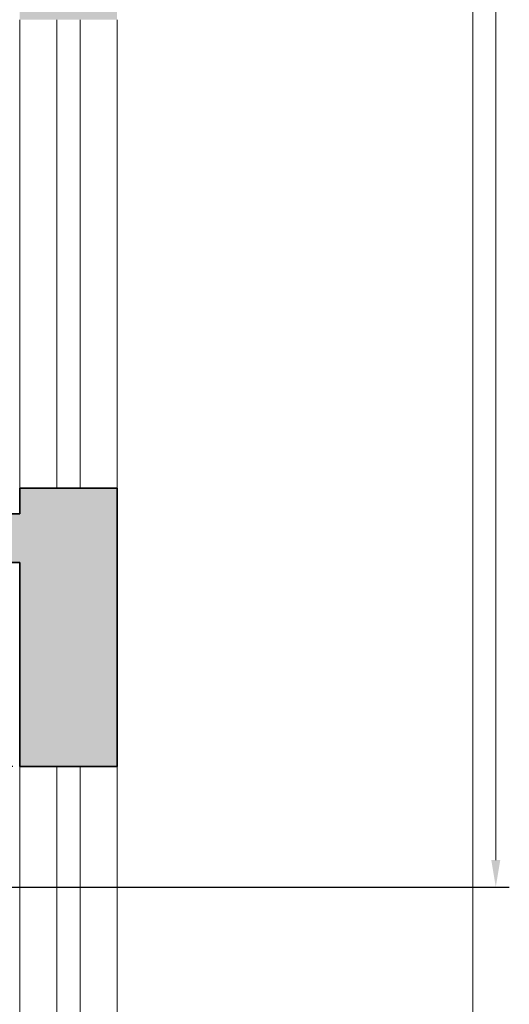
# Model space of a CAD drawing. Units: inches. Extents: x 2696 to 3240, y 1564 to 2310.
# Tile 37 of 76: x 3191 to 3236, y 1654 to 1745. Entities that reach past the tile are written whole.
import ezdxf

# ---------------------------------------------------------------- set-up
doc = ezdxf.new("R2010")
doc.units = ezdxf.units.IN
for name, color, linetype, lineweight in [('A-ANNO-DIMS', 3, 'Continuous', 18), ('A-WALL', 7, 'Continuous', 35), ('A-WALL-PATT', 9, 'Continuous', 13), ('WINDOW', 2, 'Continuous', 18)]:
    doc.layers.add(name, color=color, linetype=linetype, lineweight=lineweight)
doc.styles.add('TIMES NEW', font='times.ttf')
doc.dimstyles.new('Siddhuu', dxfattribs={"dimtxt": 6, "dimasz": 2.5, "dimexe": 1.25, "dimexo": 0.625, "dimtad": 1, "dimdec": 1, "dimlunit": 4, "dimtxsty": 'TIMES NEW', "dimcen": 2.5, "dimclrd": 256, "dimclre": 1, "dimclrt": 7, "dimadec": 0, "dimazin": 0, "dimtfac": 1, "dimtdec": 1, "dimtmove": 0, "dimatfit": 3, "dimfxl": 1, "dimtolj": 1, "dimlwd": -1, "dimarcsym": 0})

# ---------------------------------------------------------------- blocks, each defined once
blk = doc.blocks.new('WD_WIN4')
for p, q in [((-0.5, 0.5), (0.5, 0.5)), ((-0.5, 0.12), (0.5, 0.12)), ((-0.5, -0.12), (0.5, -0.12)), ((-0.5, -0.5), (0.5, -0.5))]:
    blk.add_line(p, q)
blk = doc.blocks.new('*D10')
at = {"layer": 'A-ANNO-DIMS', "color": 0, "lineweight": -2, "transparency": 16777216}
for p, q in [((3200.236, 2262.201), (3233.745, 2262.201)), ((3200.236, 1605.201), (3233.745, 1605.201))]:
    blk.add_line(p, q, dxfattribs=at)
at = {"layer": 'A-ANNO-DIMS', "color": 0, "transparency": 16777216}
blk.add_line((3232.495, 2250.201), (3232.495, 1617.201), dxfattribs=at)
for points in [[(3230.495, 2250.201), (3234.495, 2250.201), (3232.495, 2262.201)], [(3230.495, 1617.201), (3234.495, 1617.201), (3232.495, 1605.201)]]:
    blk.add_solid(points, dxfattribs=at)
at = {"layer": 'Defpoints', "color": 0, "transparency": 16777216}
for p in [(3199.611, 2262.201), (3199.611, 1605.201), (3232.495, 1605.201)]:
    blk.add_point(p, dxfattribs=at)
at = {"layer": 'A-ANNO-DIMS', "color": 0, "transparency": 16777216, "insert": (3222.714, 1933.701), "char_height": 18, "attachment_point": 5, "rotation": 90, "style": 'TIMES NEW'}
blk.add_mtext("\\A1;54'", dxfattribs=at)
blk = doc.blocks.new('*D26')
at = {"layer": 'A-ANNO-DIMS', "transparency": 16777216}
for p, q in [((3184.115, 1676.355), (3184.115, 1772.168)), ((3184.115, 1635.548), (3184.115, 1673.855))]:
    blk.add_line(p, q, dxfattribs=at)
at = {"layer": 'A-ANNO-DIMS', "color": 1, "lineweight": -2, "transparency": 16777216}
for p, q in [((3189.986, 1676.355), (3182.865, 1676.355)), ((3189.986, 1633.048), (3182.865, 1633.048))]:
    blk.add_line(p, q, dxfattribs=at)
at = {"layer": 'A-ANNO-DIMS', "transparency": 16777216}
for points in [[(3183.699, 1673.855), (3184.532, 1673.855), (3184.115, 1676.355)], [(3183.699, 1635.548), (3184.532, 1635.548), (3184.115, 1633.048)]]:
    blk.add_solid(points, dxfattribs=at)
at = {"layer": 'Defpoints', "color": 0, "transparency": 16777216}
for p in [(3184.115, 1676.355), (3190.611, 1676.355), (3190.611, 1633.048)]:
    blk.add_point(p, dxfattribs=at)
at = {"layer": 'A-ANNO-DIMS', "color": 7, "transparency": 16777216, "insert": (3180.348, 1725.511), "char_height": 6, "attachment_point": 5, "rotation": 90, "style": 'TIMES NEW'}
blk.add_mtext('\\A1;WINDOW 3\'-7 1/2" TYP.', dxfattribs=at)
blk = doc.blocks.new('*D56')
at = {"layer": 'A-ANNO-DIMS', "color": 1, "lineweight": -2, "transparency": 16777216}
for p, q in [((2966.334, 1884.201), (3235.861, 1884.201)), ((2966.334, 1665.201), (3235.861, 1665.201))]:
    blk.add_line(p, q, dxfattribs=at)
at = {"layer": 'A-ANNO-DIMS', "transparency": 16777216}
blk.add_line((3234.611, 1667.701), (3234.611, 1881.701), dxfattribs=at)
for points in [[(3234.195, 1881.701), (3235.028, 1881.701), (3234.611, 1884.201)], [(3234.195, 1667.701), (3235.028, 1667.701), (3234.611, 1665.201)]]:
    blk.add_solid(points, dxfattribs=at)
at = {"layer": 'Defpoints', "color": 0, "transparency": 16777216}
for p in [(2965.709, 1884.201), (3234.611, 1884.201), (2965.709, 1665.201)]:
    blk.add_point(p, dxfattribs=at)
at = {"layer": 'A-ANNO-DIMS', "color": 7, "transparency": 16777216, "insert": (3230.934, 1774.701), "char_height": 6, "attachment_point": 5, "rotation": 90, "style": 'TIMES NEW'}
blk.add_mtext('\\A1;18\'-3"', dxfattribs=at)

msp = doc.modelspace()

# ---------------------------------------------------------------- hatches: boundary and pattern name
at = {"layer": 'A-WALL-PATT', "transparency": 33554556}
h = msp.add_hatch(color=256, dxfattribs=at)
h.dxf.hatch_style = 1
h.paths.add_polyline_path([(2879.111, 2253.201), (2905.91, 2253.201), (2905.91, 2262.201), (2841.889, 2262.201), (2841.889, 2253.201), (2870.111, 2253.201), (2870.111, 2176.601), (2965.709, 2176.601), (2965.709, 2206.701), (2973.583, 2206.701), (2973.583, 2215.701), (2965.709, 2215.701), (2965.709, 2262.201), (2929.91, 2262.201), (2929.91, 2253.201), (2956.709, 2253.201), (2956.709, 2185.601), (2879.111, 2185.601)])
h.paths.add_polyline_path([(2782.834, 2262.201), (2745.611, 2262.201), (2745.611, 2228.729), (2754.611, 2228.729), (2754.611, 2253.201), (2782.834, 2253.201)])
h.paths.add_polyline_path([(2754.611, 2136.201), (2965.709, 2136.201), (2965.709, 2145.201), (2879.111, 2145.201), (2879.111, 2147.074), (2877.34, 2147.074), (2870.111, 2147.074), (2870.111, 2145.201), (2754.611, 2145.201), (2754.611, 2169.674), (2745.611, 2169.674), (2745.611, 2000.201), (2754.611, 2000.201), (2754.611, 2019.201), (2849.083, 2019.201), (2849.083, 2023.701), (2841.209, 2023.701), (2841.209, 2051.827), (2836.709, 2051.827), (2836.709, 2023.701), (2754.611, 2023.701), (2754.611, 2091.201), (2836.709, 2091.201), (2836.709, 2087.827), (2841.209, 2087.827), (2841.209, 2095.701), (2754.611, 2095.701)])
h.paths.add_polyline_path([(2965.709, 2136.201), (2956.709, 2136.201), (2956.709, 2023.701), (2885.083, 2023.701), (2885.083, 2019.201), (2956.709, 2019.201), (2956.709, 1950.575), (2965.709, 1950.575), (2965.709, 1980.201), (2973.583, 1980.201), (2973.583, 1989.201), (2965.709, 1989.201)])
h.paths.add_polyline_path([(2754.611, 1906.701), (2880.209, 1906.701), (2884.709, 1906.701), (2956.709, 1906.701), (2956.709, 1792.701), (2944.709, 1792.701), (2944.709, 1783.701), (2956.709, 1783.701), (2956.709, 1740.201), (2884.709, 1740.201), (2884.709, 1783.701), (2896.709, 1783.701), (2896.709, 1792.701), (2884.709, 1792.701), (2884.709, 1846.701), (2880.209, 1846.701), (2880.209, 1740.201), (2754.611, 1740.201), (2754.611, 1777.201), (2745.611, 1777.201), (2745.611, 1692.701), (2754.611, 1692.701), (2754.611, 1731.201), (2956.709, 1731.201), (2956.709, 1723.327), (2965.709, 1723.327), (2965.709, 1884.201), (2973.583, 1884.201), (2973.583, 1893.201), (2965.709, 1893.201), (2965.709, 1914.575), (2956.709, 1914.575), (2956.709, 1911.201), (2754.611, 1911.201), (2754.611, 1930.201), (2745.611, 1930.201), (2745.611, 1817.201), (2754.611, 1817.201), (2754.611, 1854.201), (2826.611, 1854.201), (2826.611, 1868.827), (2822.111, 1868.827), (2822.111, 1858.701), (2754.611, 1858.701)])
h.paths.add_polyline_path([(2965.709, 1656.201), (3008.237, 1656.201), (3008.237, 1665.201), (2965.709, 1665.201), (2965.709, 1693.327), (2956.709, 1693.327), (2956.709, 1686.201), (2934.583, 1686.201), (2934.583, 1681.701), (2956.709, 1681.701), (2956.709, 1614.201), (2896.709, 1614.201), (2896.709, 1681.701), (2904.583, 1681.701), (2904.583, 1686.201), (2892.209, 1686.201), (2892.209, 1614.201), (2858.41, 1614.201), (2858.41, 1605.201), (2965.709, 1605.201)])
h.paths.add_polyline_path([(2788.41, 1614.201), (2754.611, 1614.201), (2754.611, 1652.701), (2745.611, 1652.701), (2745.611, 1605.201), (2788.41, 1605.201)])
h.paths.add_polyline_path([(3199.611, 1633.048), (3190.611, 1633.048), (3190.611, 1614.201), (3082.611, 1614.201), (3082.611, 1665.201), (3070.237, 1665.201), (3070.237, 1656.201), (3078.111, 1656.201), (3078.111, 1605.201), (3199.611, 1605.201)])
h.paths.add_polyline_path([(3199.611, 1702.048), (3190.611, 1702.048), (3190.611, 1699.701), (3106.611, 1699.701), (3106.611, 1747.701), (3190.611, 1747.701), (3190.611, 1752.201), (3082.611, 1752.201), (3082.611, 1760.075), (3078.111, 1760.075), (3078.111, 1747.701), (3102.111, 1747.701), (3102.111, 1699.701), (3078.111, 1699.701), (3078.111, 1695.201), (3190.611, 1695.201), (3190.611, 1676.355), (3199.611, 1676.355)])
h.paths.add_polyline_path([(3199.611, 1783.201), (3190.611, 1783.201), (3190.611, 1745.355), (3199.611, 1745.355)])
h.paths.add_polyline_path([(3082.611, 1884.201), (3190.611, 1884.201), (3190.611, 1853.201), (3199.611, 1853.201), (3199.611, 1901.701), (3190.611, 1901.701), (3190.611, 1893.201), (3005.583, 1893.201), (3005.583, 1891.281), (3005.583, 1884.201), (3078.111, 1884.201), (3078.111, 1792.075), (3082.611, 1792.075)])
h.paths.add_polyline_path([(3199.611, 1994.701), (3190.611, 1994.701), (3190.611, 1989.201), (3073.709, 1989.201), (3073.709, 2034.201), (3069.209, 2034.201), (3069.209, 1989.201), (3005.583, 1989.201), (3005.583, 1980.201), (3190.611, 1980.201), (3190.611, 1971.701), (3199.611, 1971.701)])
h.paths.add_polyline_path([(3199.611, 2155.201), (3190.611, 2155.201), (3190.611, 2064.701), (3199.611, 2064.701)])
h.paths.add_polyline_path([(3190.611, 2074.701), (3106.611, 2074.701), (3106.611, 2122.701), (3190.611, 2122.701), (3190.611, 2127.201), (3082.709, 2127.201), (3082.709, 2135.075), (3073.709, 2135.075), (3073.709, 2122.701), (3102.111, 2122.701), (3102.111, 2074.701), (3069.209, 2074.701), (3069.209, 2070.201), (3190.611, 2070.201)])
h.paths.add_polyline_path([(3082.709, 2253.201), (3190.611, 2253.201), (3190.611, 2225.201), (3199.611, 2225.201), (3199.611, 2262.201), (3073.709, 2262.201), (3073.709, 2215.701), (3035.583, 2215.701), (3035.583, 2206.701), (3073.709, 2206.701), (3073.709, 2171.075), (3082.709, 2171.075)])

# ---------------------------------------------------------------- linework, layer by layer
at = {"layer": 'A-WALL'}
for p, q in [((3190.611, 1699.701), (3190.611, 1702.048)), ((3190.611, 1702.048), (3199.611, 1702.048)), ((3199.611, 1676.355), (3199.611, 1702.048)), ((3106.611, 1699.701), (3190.611, 1699.701)), ((3078.111, 1695.201), (3190.611, 1695.201)), ((3190.611, 1676.355), (3190.611, 1695.201)), ((3190.611, 1676.355), (3199.611, 1676.355))]:
    msp.add_line(p, q, dxfattribs=at)

# ---------------------------------------------------------------- block references
at = {"layer": 'WINDOW', "xscale": 43.30708661417323, "yscale": 8.999999999999545, "zscale": 43.30708661417323}
for p, rotation in [((3195.111, 1723.701), 270.0000000000006), ((3195.111, 1654.701), 90)]:
    msp.add_blockref('WD_WIN4', p, dxfattribs=dict(at, rotation=rotation))

# ---------------------------------------------------------------- dimensions: what is measured, and where the dimension line sits
at = {"layer": 'A-ANNO-DIMS'}
for base, p1, p2, text, override, picture, middle in [((3232.495, 1605.201), (3199.611, 2262.201), (3199.611, 1605.201), "54'", {"dimtxt": 18, "dimasz": 12, "dimclrd": 0, "dimclre": 0, "dimclrt": 0}, '*D10', (3222.714, 1933.701)), ((3184.115, 1676.355), (3190.611, 1633.048), (3190.611, 1676.355), 'WINDOW <> TYP.', {"dimdec": 1, "dimlfac": 1, "dimrnd": 0, "dimzin": 1, "dimdsep": 46, "dimlunit": 4, "dimfrac": 2}, '*D26', (3180.348, 1725.511))]:
    dim = msp.add_linear_dim(base=base, p1=p1, p2=p2, angle=90, text=text, dimstyle='Siddhuu', override=override, dxfattribs=at)
    dim.commit()
    dim.dimension.update_dxf_attribs({"geometry": picture, "text_midpoint": middle})
dim = msp.add_linear_dim(base=(3234.611, 1884.201), p1=(2965.709, 1665.201), p2=(2965.709, 1884.201), angle=90, dimstyle='Siddhuu', override={"dimdec": 1, "dimlfac": 1, "dimrnd": 0, "dimzin": 1, "dimdsep": 46, "dimlunit": 4, "dimfrac": 2}, dxfattribs=at)
dim.commit()
dim.dimension.update_dxf_attribs({"geometry": '*D56', "text_midpoint": (3230.934, 1774.701)})

doc.saveas('drawing.dxf')
